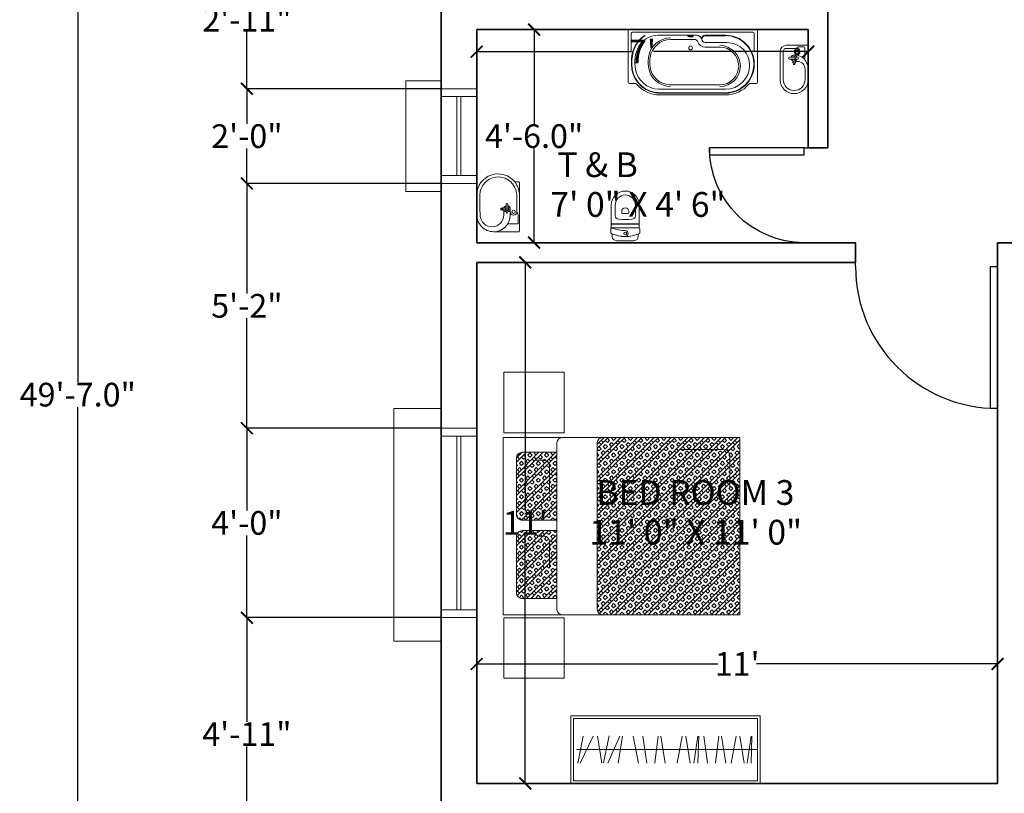
# Model space of a CAD drawing. Units: inches. Extents: x 844 to 2234, y 346 to 1084.
# Tile 48 of 93: x 1590 to 1840, y 632 to 828. Entities that reach past the tile are written whole.
import ezdxf

# ---------------------------------------------------------------- set-up
doc = ezdxf.new("R2010")
doc.units = ezdxf.units.IN
doc.header["$MEASUREMENT"] = 0
for name, color, linetype, lineweight in [('A-ANNO-DIMS', 2, 'Continuous', 18), ('A-AREA-IDEN', 7, 'Continuous', 18), ('A-FLOR-FIXT', 8, 'Continuous', 18), ('A-WALL', 7, 'Continuous', 35), ('beds', 130, 'Continuous', 18), ('doors', 170, 'Continuous', 25), ('furniture', 8, 'Continuous', 18), ('windows', 1, 'Continuous', 18)]:
    doc.layers.add(name, color=color, linetype=linetype, lineweight=lineweight)
doc.styles.get("Standard").update_dxf_attribs({"font": 'arial.ttf'})
doc.dimstyles.get("Standard").update_dxf_attribs({"dimtxt": 6, "dimasz": 3, "dimexe": 0.18, "dimexo": 0.0625, "dimgap": 0.09, "dimtad": 0, "dimtih": 1, "dimtoh": 1, "dimdec": 1, "dimzin": 0, "dimdsep": 46, "dimlunit": 3, "dimtxsty": 'Standard', "dimblk": 'ARCHTICK', "dimcen": 0.09, "dimadec": 0, "dimazin": 0, "dimtfac": 1, "dimtdec": 1, "dimtofl": 0, "dimtmove": 0, "dimatfit": 3, "dimfxl": 1, "dimtolj": 1, "dimtzin": 0, "dimarcsym": 0})
pattern_1 = [(135, (-1377.70473, -125.71507), (-0.070710678, -0.070710678), []), (135, (-1377.68705, -125.69739), (-0.070710678, -0.070710678), []), (45, (-1377.70473, -125.71507), (-0.070710678, 0.070710678), [-0.025, 0.025]), (45, (-1377.72241, -125.69739), (-0.070710678, 0.070710678), [-0.025, 0.025]), (45, (-1377.74009, -125.67972), (-0.070710678, 0.070710678), [0.025, -0.025]), (45, (-1377.75776, -125.66204), (-0.070710678, 0.070710678), [0.025, -0.025]), (135, (-1377.66938, -125.67972), (-0.070710678, -0.070710678), [0.025, -0.025]), (135, (-1377.6517, -125.66204), (-0.070710678, -0.070710678), [0.025, -0.025])]

# ---------------------------------------------------------------- blocks, each defined once
blk = doc.blocks.new('*U2')
for p, q in [((0, 0), (0, -6)), ((36, 0), (36, -6))]:
    blk.add_line(p, q)
blk.add_lwpolyline([(0, 0), (0, 36), (1.75, 36), (1.75, 0)], close=True)
blk.add_arc((0, 0), 36, 0, 90)
blk = doc.blocks.new('*U4')
for p, q in [((0, 0), (0, -6)), ((24, 0), (24, -6))]:
    blk.add_line(p, q)
blk.add_lwpolyline([(0, 0), (0, 24), (1.75, 24), (1.75, 0)], close=True)
blk.add_arc((0, 0), 24, 0, 90)
blk = doc.blocks.new('MAT-P10')
h = blk.add_hatch()
h.set_pattern_fill('BOX', color=256, scale=0.1, angle=45, style=0)
h.set_pattern_definition(pattern_1)
h.paths.add_polyline_path([(-0.1565, 1.4605), (0.417, 1.4605), (0.417, 1.7513, 0.414214), (0.367, 1.8013), (-0.1065, 1.8013, 0.414214), (-0.1565, 1.7513)])
h.paths.add_polyline_path([(0.5052, 1.4604), (1.0792, 1.4604), (1.0792, 1.7513, 0.414214), (1.0292, 1.8013), (0.5552, 1.8013, 0.414214), (0.5052, 1.7513)])
h = blk.add_hatch()
h.set_pattern_fill('BOX', color=256, scale=0.1, angle=45, style=0)
h.set_pattern_definition(pattern_1)
edge = h.paths.add_edge_path()
edge.add_line((1.2049, -0.085), (1.2049, 1.0625))
edge.add_ellipse((1.1608, 1.0627), major_axis=(0, 0.0568), ratio=0.776379, start_angle=270, end_angle=360)
edge.add_line((1.1608, 1.1195), (-0.251, 1.1195))
edge.add_ellipse((-0.251, 1.0627), major_axis=(0, 0.0568), ratio=0.776379, start_angle=0, end_angle=88.13958)
edge.add_line((-0.2951, 1.0641), (-0.2951, -0.085))
edge.add_line((-0.2951, -0.085), (1.2049, -0.085))
for p, q in [((-0.251, 1.4605), (1.1608, 1.4604)), ((-0.251, 1.1195), (1.1608, 1.1195)), ((1.1017, 0.406), (1.1017, 0.0572)), ((1.0576, 0.0004), (0.7754, 0.0004))]:
    blk.add_line(p, q)
for points in [[(1.2049, -0.085), (-0.2951, -0.085), (-0.2951, 1.9151), (1.2049, 1.915)], [(-0.8301, 1.9091), (-0.3191, 1.9091), (-0.3191, 1.3981), (-0.8301, 1.3981)], [(1.2441, 1.9091), (1.755, 1.9091), (1.755, 1.3981), (1.2441, 1.3981)]]:
    blk.add_lwpolyline(points, close=True)
for points in [[(0.417, 1.4604), (0.417, 1.7513, 0.414214), (0.367, 1.8013), (-0.1065, 1.8013, 0.414214), (-0.1565, 1.7513), (-0.1565, 1.4604)], [(1.0792, 1.4603), (1.0792, 1.7513, 0.414214), (1.0292, 1.8013), (0.5552, 1.8013, 0.414214), (0.5052, 1.7513), (0.5052, 1.4604)], [(0.3702, 1.6242), (0.3702, 1.5715, -0.414214), (0.3202, 1.5215), (0.1113, 1.5215)], [(1.0117, 1.6438), (1.0117, 1.5715, -0.414214), (0.9617, 1.5215), (0.7528, 1.5215)]]:
    blk.add_lwpolyline(points, format="xyb")
at = {"extrusion": (0, 0, -1)}
for centre, start_param, end_param in [((-0.251, 1.4036), 4.712389, 6.283185), ((1.1608, 1.4036), 0, 1.570796), ((-0.251, 1.0627), 4.712389, 6.283185), ((1.1608, 1.0627), 0, 1.570796), ((1.0576, 0.0572), 1.570796, 3.141593), ((1.0576, 0.0572), 1.570796, 3.141593)]:
    blk.add_ellipse(centre, major_axis=(0, 0.0568), ratio=0.776379, start_param=start_param, end_param=end_param, dxfattribs=at)
blk = doc.blocks.new('A$C7A17768A')
for p, q in [((-2.8, 0), (0, 0)), ((-2.8, -1), (-2.8, 0)), ((0, -1), (0, 0)), ((-2.76, -0.04), (-0.04, -0.04)), ((-2.76, -0.96), (-2.76, -0.04)), ((-0.04, -0.96), (-0.04, -0.04)), ((-2.617, -0.3), (-2.694, -0.7)), ((-2.66, -0.7), (-2.466, -0.3)), ((-2.403, -0.3), (-2.342, -0.7)), ((-2.229, -0.296), (-2.317, -0.696)), ((-2.074, -0.3), (-2.25, -0.7)), ((-2.096, -0.7), (-2.033, -0.3)), ((-1.875, -0.3), (-1.796, -0.7)), ((-1.732, -0.3), (-1.675, -0.7)), ((-1.555, -0.7), (-1.507, -0.3)), ((-1.467, -0.3), (-1.403, -0.7)), ((-1.227, -0.7), (-1.151, -0.3)), ((-1.098, -0.3), (-1.034, -0.7)), ((-0.98, -0.7), (-0.921, -0.3)), ((-0.908, -0.3), (-0.919, -0.7)), ((-0.834, -0.3), (-0.777, -0.7)), ((-0.657, -0.7), (-0.61, -0.3)), ((-0.57, -0.3), (-0.505, -0.7)), ((-0.429, -0.7), (-0.353, -0.3)), ((-0.301, -0.3), (-0.237, -0.7)), ((-0.192, -0.7), (-0.133, -0.3)), ((-0.12, -0.3), (-0.131, -0.7)), ((-0.04, -0.5), (-2.716, -0.5)), ((-2.8, -1), (0, -1)), ((-2.76, -0.96), (-0.04, -0.96))]:
    blk.add_line(p, q)
blk = doc.blocks.new('2SABICO')
at = {"color": 0, "linetype": 'ByBlock'}
for p, q in [((0.478, 0.195), (0.089, 0.195)), ((0.478, 0.152), (0.089, 0.152)), ((0, 0.106), (0, 0)), ((0, 0), (0, -0.18)), ((0.043, -0.039), (0.043, 0.106)), ((0.135, 0), (0.135, -0.003)), ((0.168, 0.064), (0.168, -0.015)), ((0.192, 0.064), (0.192, -0.015)), ((0.221, 0.012), (0.222, 0.012)), ((0.223, 0.016), (0.223, -0.016)), ((0.224, 0.017), (0.245, 0.017)), ((0.246, 0.016), (0.246, -0.016)), ((0.25, 0.014), (0.246, 0.014)), ((0.26, 0.01), (0.268, 0.01)), ((0.268, -0.01), (0.268, 0.01)), ((0.268, 0.01), (0.269, 0.009)), ((0.269, -0.009), (0.269, 0.009)), ((0.023, -0.057), (0.023, -0.135)), ((0.135, 0), (0.135, -0.039)), ((0.168, -0.015), (0.192, -0.015)), ((0.168, -0.015), (0.168, -0.046)), ((0.192, -0.015), (0.192, -0.046)), ((0.221, -0.012), (0.222, -0.012)), ((0.224, -0.017), (0.245, -0.017)), ((0.225, -0.017), (0.225, -0.047)), ((0.25, -0.014), (0.246, -0.014)), ((0.26, -0.01), (0.268, -0.01)), ((0.268, -0.01), (0.269, -0.009)), ((0.015, -0.195), (0.478, -0.195)), ((0.038, -0.15), (0.179, -0.15)), ((0.33, -0.152), (0.478, -0.152))]:
    blk.add_line(p, q, dxfattribs=at)
for radius in [0.035, 0.023]:
    blk.add_circle((0.089, -0.039), radius, dxfattribs=at)
for centre, radius, start, end in [((0.089, 0.106), 0.089, 90, 180), ((0.089, 0.106), 0.046, 90, 180), ((0.478, 0), 0.195, 270, 90), ((0.478, 0), 0.152, 270, 90), ((0.18, 0), 0.045, 105.6643, 180), ((0.18, 0), 0.042, 106.8152, 252.6853), ((0.18, 0), 0.0235, 121.1327, 237.8651), ((0.18, 0.064), 0.0121, 0, 180), ((0.18, 0), 0.045, 17.0576, 74.3357), ((0.18, 0), 0.042, 287.3147, 73.1848), ((0.18, 0), 0.0235, 302.1349, 58.8673), ((0.221, 0.013), 0.001, 197.9471, 270), ((0.222, 0.013), 0.001, 270, 0), ((0.224, 0.016), 0.001, 90, 180), ((0.245, 0.016), 0.001, 0, 90), ((0.25, 0), 0.0143, 270, 90), ((0.041, -0.057), 0.018, 99.5941, 180), ((0.038, -0.135), 0.015, 180, 270), ((0.037, -0.033), 0.006, 279.5941, 0), ((0.089, -0.039), 0.046, 180, 360), ((0.326, -0.003), 0.191, 180, 270), ((0.18, -0.046), 0.0125, 180, 0), ((0.179, -0.14), 0.01, 270, 42.9682), ((0.221, -0.013), 0.001, 90, 162.0529), ((0.222, -0.013), 0.001, 0, 90), ((0.224, -0.016), 0.001, 180, 270), ((0.33, -0.047), 0.105, 180, 270), ((0.245, -0.016), 0.001, 270, 0), ((0.015, -0.18), 0.015, 180, 270)]:
    blk.add_arc(centre, radius, start, end, dxfattribs=at)
blk = doc.blocks.new('2SAINCO')
at = {"color": 0, "linetype": 'ByBlock'}
for p, q in [((0.06, 0.181), (0.085, 0.181)), ((0.114, 0.203), (0.165, 0.203)), ((0.496, 0.195), (0.178, 0.195)), ((0.18, -0.188), (0.18, 0.188)), ((0.231, 0.185), (0.231, -0.185)), ((0.234, 0.185), (0.234, -0.185)), ((0.496, 0.14), (0.347, 0.14)), ((0, -0.121), (0, 0.121)), ((0.394, 0.05), (0.407, 0.05)), ((0.394, -0.05), (0.407, -0.05)), ((0.06, -0.181), (0.085, -0.181)), ((0.114, -0.201), (0.165, -0.201)), ((0.114, -0.203), (0.165, -0.203)), ((0.496, -0.195), (0.178, -0.195)), ((0.496, -0.14), (0.347, -0.14))]:
    blk.add_line(p, q, dxfattribs=at)
blk.add_circle((0.1, 0), 0.02, dxfattribs=at)
for centre, radius, start, end in [((0.06, 0.121), 0.06, 90, 180), ((0.517, 0), 0.46, 155.909, 204.091), ((0.085, 0.196), 0.015, 270, 344.534), ((0.114, 0.188), 0.015, 90, 164.534), ((0.165, 0.188), 0.015, 0, 90), ((0.221, 0.185), 0.01, 0, 90), ((0.224, 0.185), 0.01, 0, 90), ((0.347, 0.09), 0.05, 90, 177.3546), ((0.496, 0), 0.195, 270, 90), ((0.496, 0), 0.14, 270, 90), ((0.1, 0), 0.0405, 360, 180), ((0.517, 0), 0.458, 180, 204.67), ((0.66, 0.008), 0.52, 180.891, 201.3823), ((2.295, 0), 2, 177.3546, 182.6454), ((0.677, 0), 0.3, 172.9459, 187.0541), ((0.394, 0.035), 0.015, 90, 172.9459), ((0.407, 0), 0.05, 270, 90), ((0.06, -0.121), 0.06, 180, 270), ((0.347, -0.09), 0.05, 182.6454, 270), ((0.394, -0.035), 0.015, 187.0541, 270), ((0.085, -0.196), 0.015, 15.466, 90), ((0.114, -0.188), 0.015, 195.466, 270), ((0.114, -0.188), 0.013, 195.466, 270), ((0.165, -0.188), 0.013, 270, 30), ((0.165, -0.188), 0.015, 270, 0), ((0.221, -0.185), 0.01, 270, 0), ((0.224, -0.185), 0.01, 270, 0)]:
    blk.add_arc(centre, radius, start, end, dxfattribs=at)
blk = doc.blocks.new('2SABACO')
at = {"color": 0}
for p, q in [((1.341, 0.831), (0.407, 0.831)), ((1.341, 0.91), (0.429, 0.91)), ((1.341, 0.885), (0.429, 0.885)), ((1.341, 0.879), (0.429, 0.879)), ((-0.015, 0.735), (-0.015, 0.015)), ((0, 0.75), (0.08, 0.75)), ((1.263, 0.769), (0.562, 0.769)), ((1.77, 0.75), (1.69, 0.75)), ((1.785, 0.015), (1.785, 0.735)), ((0.03, 0.302), (0.03, 0.053)), ((1.74, 0.053), (1.74, 0.286)), ((0.578, 0.139), (0.911, 0.139)), ((1.263, 0.245), (1.06, 0.245)), ((1.363, 0.181), (1.06, 0.181)), ((0, 0), (1.77, 0)), ((0.048, 0.035), (1.722, 0.035)), ((0.401, 0.08), (0.942, 0.08)), ((1.343, 0.086), (1.06, 0.086)), ((1.343, 0.079), (1.06, 0.079))]:
    blk.add_line(p, q, dxfattribs=at)
blk.add_circle((0.855, 0.256), 0.026, dxfattribs=at)
for centre, radius, start, end in [((0.428, 0.49), 0.395, 98.9726, 181.1954), ((0.428, 0.49), 0.389, 98.9726, 181.2301), ((0.425, 0.49), 0.342, 93.1008, 168.0202), ((0.429, 0.48), 0.43, 90, 139.2943), ((0.429, 0.48), 0.405, 90, 98.9726), ((0.429, 0.48), 0.399, 90, 98.9726), ((1.341, 0.48), 0.43, 40.7057, 90), ((1.341, 0.485), 0.401, 359.4627, 90), ((1.341, 0.485), 0.394, 3.5237, 90), ((1.341, 0.495), 0.336, 0, 90), ((0, 0.735), 0.015, 90, 180), ((0.08, 0.78), 0.03, 270, 319.2943), ((0.578, 0.481), 0.311, 90, 172.609), ((0.578, 0.481), 0.288, 93.3767, 172.609), ((1.263, 0.507), 0.285, 270, 90), ((1.263, 0.507), 0.262, 270, 90), ((1.69, 0.78), 0.03, 220.7057, 270), ((1.77, 0.735), 0.015, 0, 90), ((0.559, 0.454), 0.48, 163.1286, 202.3619), ((0.559, 0.454), 0.528, 177.0415, 202.3619), ((0.559, 0.454), 0.521, 177.0156, 202.3619), ((0.79, 0.454), 0.525, 172.609, 180), ((0.79, 0.454), 0.525, 180, 187.391), ((0.79, 0.454), 0.502, 172.609, 180), ((0.79, 0.454), 0.502, 180, 187.391), ((1.343, 0.477), 0.392, 270, 4.5675), ((1.343, 0.477), 0.398, 270, 0.539), ((1.363, 0.495), 0.314, 270, 2.2815), ((0.042, 0.302), 0.0116, 16.3184, 180.0001), ((0.578, 0.427), 0.311, 187.391, 270), ((0.578, 0.427), 0.288, 187.391, 270), ((1.718, 0.286), 0.0222, 0, 152.9966), ((0.401, 0.389), 0.357, 202.3619, 239.8287), ((0.401, 0.389), 0.351, 202.3619, 239.2093), ((0.401, 0.389), 0.309, 202.3619, 270), ((0.911, 0.183), 0.045, 270, 341.2369), ((1.06, 0.133), 0.112, 90, 161.2369), ((1.06, 0.133), 0.0475, 90, 270), ((0, 0.015), 0.015, 180, 270), ((0.048, 0.053), 0.018, 180, 270), ((0.559, 0.454), 0.48, 250.7818, 251.0555), ((0.821, 0.092), 0.00282, 119.7759, 180), ((0.821, 0.092), 0.00282, 180, 240.2241), ((0.837, 0.064), 0.0347, 103.3326, 119.7759), ((0.835, 0.025), 0.071, 96.5949, 102.1924), ((0.837, 0.12), 0.0347, 240.2241, 256.6674), ((0.847, -0.08), 0.177, 92.7417, 96.5949), ((0.848, 0.02), 0.0808, 95.6065, 103.3326), ((0.848, 0.164), 0.0808, 256.6674, 264.3935), ((0.855, -0.252), 0.349, 90, 92.7417), ((0.855, -0.053), 0.153, 90, 95.6065), ((0.855, 0.237), 0.153, 264.3935, 270), ((0.855, -0.053), 0.153, 84.3935, 90), ((0.855, -0.252), 0.349, 87.2583, 90), ((0.855, 0.237), 0.153, 270, 275.6065), ((0.862, 0.02), 0.0808, 76.6674, 84.3935), ((0.862, 0.164), 0.0808, 275.6065, 283.3326), ((0.863, -0.08), 0.177, 83.4051, 87.2583), ((0.873, 0.064), 0.0347, 60.2241, 76.6674), ((0.873, 0.12), 0.0347, 283.3326, 299.7759), ((0.875, 0.025), 0.071, 77.8076, 83.4051), ((0.889, 0.092), 0.00282, 360, 60.2241), ((0.889, 0.092), 0.00282, 299.7759, 360), ((0.942, 0.145), 0.065, 270, 349.4977), ((1.06, 0.133), 0.054, 180, 270), ((1.722, 0.053), 0.018, 270, 0), ((1.77, 0.015), 0.015, 270, 0)]:
    blk.add_arc(centre, radius, start, end, dxfattribs=at)
blk = doc.blocks.new('2SALACO2')
at = {"color": 0}
for p, q in [((0, 0), (-0.392, 0)), ((0.28, 0), (0, 0)), ((-0.402, -0.01), (-0.402, -0.36)), ((-0.293, -0.026), (-0.293, -0.15)), ((-0.283, -0.016), (-0.166, -0.016)), ((-0.169, -0.128), (-0.085, -0.128)), ((-0.112, -0.035), (-0.133, -0.035)), ((-0.124, -0.035), (0.09, -0.035)), ((0.29, -0.01), (0.29, -0.064)), ((-0.102, -0.219), (-0.169, -0.219)), ((-0.1, -0.161), (-0.131, -0.161)), ((-0.1, -0.186), (-0.131, -0.186)), ((-0.102, -0.217), (-0.102, -0.234)), ((-0.07, -0.216), (-0.101, -0.216)), ((-0.07, -0.235), (-0.101, -0.235)), ((-0.1, -0.161), (-0.1, -0.186)), ((-0.021, -0.161), (-0.1, -0.161)), ((-0.021, -0.186), (-0.1, -0.186)), ((-0.098, -0.214), (-0.098, -0.216)), ((-0.097, -0.239), (-0.098, -0.241)), ((-0.098, -0.241), (-0.098, -0.248)), ((-0.098, -0.241), (-0.073, -0.241)), ((-0.073, -0.248), (-0.098, -0.248)), ((-0.097, -0.235), (-0.097, -0.239)), ((-0.074, -0.239), (-0.097, -0.239)), ((-0.097, -0.248), (-0.097, -0.256)), ((-0.073, -0.256), (-0.097, -0.256)), ((-0.097, -0.256), (-0.094, -0.257)), ((-0.077, -0.257), (-0.094, -0.257)), ((-0.073, -0.256), (-0.077, -0.257)), ((-0.074, -0.235), (-0.074, -0.239)), ((-0.074, -0.239), (-0.073, -0.241)), ((-0.073, -0.214), (-0.073, -0.216)), ((-0.073, -0.241), (-0.073, -0.248)), ((-0.073, -0.248), (-0.073, -0.256)), ((-0.069, -0.217), (-0.069, -0.234))]:
    blk.add_line(p, q, dxfattribs=at)
blk.add_lwpolyline([(-0.402, -0.36, 0.423787), (-0.161, -0.593, 0.423787)], format="xyb", dxfattribs=at)
blk.add_circle((-0.124, -0.081), 0.023, dxfattribs=at)
for centre, radius, start, end in [((-0.392, -0.01), 0.01, 90, 180), ((0.28, -0.01), 0.01, 0, 90), ((-0.169, -0.36), 0.233, 90, 180), ((-0.283, -0.026), 0.01, 90, 180), ((-0.124, -0.081), 0.0462, 90, 270), ((-0.166, -0.046), 0.03, 31.2573, 90), ((-0.133, -0.026), 0.009, 211.2573, 270), ((-0.085, -0.173), 0.042, 16.8152, 162.6853), ((-0.085, -0.173), 0.0458, 15.3964, 90), ((0.09, -0.29), 0.255, 68.9449, 90), ((0.105, -0.295), 0.255, 271.0077, 72.4499), ((0.105, -0.297), 0.297, 271.4871, 51.4524), ((0.105, -0.297), 0.297, 51.4524, 87.1707), ((-0.169, -0.383), 0.164, 90, 265.4963), ((-0.285, -0.15), 0.008, 180, 299.1062), ((-0.131, -0.173), 0.0125, 90, 270), ((-0.085, -0.173), 0.042, 197.3147, 343.1848), ((-0.085, -0.173), 0.0235, 31.1327, 147.8651), ((-0.085, -0.173), 0.0235, 212.1349, 328.8673), ((-0.101, -0.217), 0.001, 90, 180), ((-0.101, -0.234), 0.001, 180, 270), ((-0.085, -0.173), 0.0458, 289.9182, 344.6036), ((-0.07, -0.217), 0.001, 0, 90), ((-0.07, -0.234), 0.001, 270, 0), ((-0.021, -0.173), 0.0121, 270, 90), ((0.021, 4.449), 5, 267.6742, 271.0081), ((-0.017, 4.405), 5, 268.3511, 271.4874)]:
    blk.add_arc(centre, radius, start, end, dxfattribs=at)
blk = doc.blocks.new('_ArchTick')
at = {"color": 0, "linetype": 'ByBlock', "const_width": 0.15}
blk.add_lwpolyline([(-0.5, -0.5), (0.5, 0.5)], dxfattribs=at)
blk = doc.blocks.new('*D67')
at = {"layer": 'A-ANNO-DIMS', "color": 0, "lineweight": -2, "transparency": 16777216}
for p, q in [((1714.3, 766.46), (1718.59, 766.46)), ((1718.41, 766.46), (1718.41, 703.56)), ((1718.41, 634.46), (1718.41, 697.35)), ((1714.3, 634.46), (1718.59, 634.46))]:
    blk.add_line(p, q, dxfattribs=at)
at = {"layer": 'Defpoints', "color": 0, "transparency": 16777216}
for p in [(1714.24, 766.46), (1714.24, 634.46), (1718.41, 634.46)]:
    blk.add_point(p, dxfattribs=at)
at = {"layer": 'A-ANNO-DIMS', "color": 0, "lineweight": -2, "transparency": 16777216, "xscale": 3, "yscale": 3, "zscale": 3}
for p, rotation in [((1718.41, 766.46), 90), ((1718.41, 634.46), 270)]:
    blk.add_blockref('_ArchTick', p, dxfattribs=dict(at, rotation=rotation))
at = {"layer": 'A-ANNO-DIMS', "color": 0, "transparency": 16777216, "insert": (1718.41, 700.46), "char_height": 6, "attachment_point": 5}
blk.add_mtext("\\A1;11'", dxfattribs=at)
blk = doc.blocks.new('*D68')
at = {"layer": 'A-ANNO-DIMS', "color": 0, "lineweight": -2, "transparency": 16777216}
for p, q in [((1706.1, 664.78), (1706.1, 664.9)), ((1706.1, 664.72), (1767.2, 664.72)), ((1838.1, 664.72), (1777, 664.72)), ((1838.1, 664.78), (1838.1, 664.9))]:
    blk.add_line(p, q, dxfattribs=at)
at = {"layer": 'Defpoints', "color": 0, "transparency": 16777216}
for p in [(1706.1, 664.72), (1838.1, 664.72), (1838.1, 664.72)]:
    blk.add_point(p, dxfattribs=at)
at = {"layer": 'A-ANNO-DIMS', "color": 0, "lineweight": -2, "transparency": 16777216, "xscale": 3, "yscale": 3, "zscale": 3, "rotation": 180}
blk.add_blockref('_ArchTick', (1706.1, 664.72), dxfattribs=at)
at = {"layer": 'A-ANNO-DIMS', "color": 0, "lineweight": -2, "transparency": 16777216, "xscale": 3, "yscale": 3, "zscale": 3}
blk.add_blockref('_ArchTick', (1838.1, 664.72), dxfattribs=at)
at = {"layer": 'A-ANNO-DIMS', "color": 0, "transparency": 16777216, "insert": (1772.1, 664.72), "char_height": 6, "attachment_point": 5}
blk.add_mtext("\\A1;11'", dxfattribs=at)
blk = doc.blocks.new('*D63')
at = {"layer": 'A-ANNO-DIMS', "color": 0, "lineweight": -2, "transparency": 16777216}
for p, q in [((1733.04, 825.46), (1720.47, 825.46)), ((1720.65, 825.46), (1720.65, 801.61)), ((1720.65, 771.46), (1720.65, 795.3)), ((1733.04, 771.46), (1720.47, 771.46))]:
    blk.add_line(p, q, dxfattribs=at)
at = {"layer": 'Defpoints', "color": 0, "transparency": 16777216}
for p in [(1733.1, 825.46), (1720.65, 771.46), (1733.1, 771.46)]:
    blk.add_point(p, dxfattribs=at)
at = {"layer": 'A-ANNO-DIMS', "color": 0, "lineweight": -2, "transparency": 16777216, "xscale": 3, "yscale": 3, "zscale": 3}
for p, rotation in [((1720.65, 825.46), 90), ((1720.65, 771.46), 270)]:
    blk.add_blockref('_ArchTick', p, dxfattribs=dict(at, rotation=rotation))
at = {"layer": 'A-ANNO-DIMS', "color": 0, "transparency": 16777216, "insert": (1720.65, 798.46), "char_height": 6, "attachment_point": 5}
blk.add_mtext('\\A1;4\'-6.0"', dxfattribs=at)
blk = doc.blocks.new('*D64')
at = {"layer": 'A-ANNO-DIMS', "color": 0, "lineweight": -2, "transparency": 16777216}
for p, q in [((1706.1, 823.41), (1706.1, 819.69)), ((1790.1, 823.41), (1790.1, 819.69)), ((1706.1, 819.87), (1745.27, 819.87)), ((1790.1, 819.87), (1750.93, 819.87))]:
    blk.add_line(p, q, dxfattribs=at)
at = {"layer": 'Defpoints', "color": 0, "transparency": 16777216}
for p in [(1706.1, 823.47), (1790.1, 823.47), (1706.1, 819.87)]:
    blk.add_point(p, dxfattribs=at)
at = {"layer": 'A-ANNO-DIMS', "color": 0, "lineweight": -2, "transparency": 16777216, "xscale": 3, "yscale": 3, "zscale": 3, "rotation": 180}
blk.add_blockref('_ArchTick', (1706.1, 819.87), dxfattribs=at)
at = {"layer": 'A-ANNO-DIMS', "color": 0, "lineweight": -2, "transparency": 16777216, "xscale": 3, "yscale": 3, "zscale": 3}
blk.add_blockref('_ArchTick', (1790.1, 819.87), dxfattribs=at)
at = {"layer": 'A-ANNO-DIMS', "color": 0, "transparency": 16777216, "insert": (1748.1, 819.87), "char_height": 6, "attachment_point": 5}
blk.add_mtext("\\A1;7'", dxfattribs=at)
blk = doc.blocks.new('*D87')
at = {"layer": 'A-ANNO-DIMS', "color": 0, "lineweight": -2, "transparency": 16777216}
for p, q in [((1697.04, 1030.46), (1604.81, 1030.46)), ((1604.99, 1030.46), (1604.99, 736.11)), ((1604.99, 435.46), (1604.99, 729.8)), ((1697.04, 435.46), (1604.81, 435.46))]:
    blk.add_line(p, q, dxfattribs=at)
at = {"layer": 'Defpoints', "color": 0, "transparency": 16777216}
for p in [(1697.1, 1030.46), (1604.99, 435.46), (1697.1, 435.46)]:
    blk.add_point(p, dxfattribs=at)
at = {"layer": 'A-ANNO-DIMS', "color": 0, "lineweight": -2, "transparency": 16777216, "xscale": 3, "yscale": 3, "zscale": 3}
for p, rotation in [((1604.99, 1030.46), 90), ((1604.99, 435.46), 270)]:
    blk.add_blockref('_ArchTick', p, dxfattribs=dict(at, rotation=rotation))
at = {"layer": 'A-ANNO-DIMS', "color": 0, "transparency": 16777216, "insert": (1604.99, 732.96), "char_height": 6, "attachment_point": 5}
blk.add_mtext('\\A1;49\'-7.0"', dxfattribs=at)
blk = doc.blocks.new('WIN-48IN')
for p, q in [((0, 9), (0, 21)), ((0, 21), (59, 21)), ((59, 9), (59, 21)), ((6, 9), (0, 9)), ((54, 9), (6, 9)), ((6, 9), (6, 0)), ((8, 9), (8, 0)), ((52, 0), (52, 9)), ((54, 0), (54, 9)), ((54, 9), (59, 9)), ((8, 5), (52, 5)), ((8, 4), (52, 4)), ((6, 0), (54, 0))]:
    blk.add_line(p, q)
blk = doc.blocks.new('WIN-24IN')
for p, q in [((9, 28), (0, 28)), ((0, 0), (0, 28)), ((9, 26), (9, 28)), ((18, 26), (9, 26)), ((9, 26), (9, 2)), ((18, 2), (18, 26)), ((18, 24), (9, 24)), ((13, 4), (13, 24)), ((14, 4), (14, 24)), ((9, 4), (18, 4)), ((9, 2), (18, 2)), ((9, 2), (9, 0)), ((9, 0), (0, 0))]:
    blk.add_line(p, q)
blk = doc.blocks.new('*D163')
at = {"layer": 'A-ANNO-DIMS', "color": 0, "lineweight": -2, "transparency": 16777216}
for p, q in [((1697.04, 676.46), (1647.67, 676.46)), ((1647.85, 676.46), (1647.85, 650.06)), ((1647.85, 617.46), (1647.85, 643.85)), ((1697.04, 617.46), (1647.67, 617.46))]:
    blk.add_line(p, q, dxfattribs=at)
at = {"layer": 'Defpoints', "color": 0, "transparency": 16777216}
for p in [(1647.85, 676.46), (1697.1, 676.46), (1697.1, 617.46)]:
    blk.add_point(p, dxfattribs=at)
at = {"layer": 'A-ANNO-DIMS', "color": 0, "lineweight": -2, "transparency": 16777216, "xscale": 3, "yscale": 3, "zscale": 3}
for p, rotation in [((1647.85, 676.46), 90), ((1647.85, 617.46), 270)]:
    blk.add_blockref('_ArchTick', p, dxfattribs=dict(at, rotation=rotation))
at = {"layer": 'A-ANNO-DIMS', "color": 0, "transparency": 16777216, "insert": (1647.85, 646.96), "char_height": 6, "attachment_point": 5}
blk.add_mtext('\\A1;4\'-11"', dxfattribs=at)
blk = doc.blocks.new('*D164')
at = {"layer": 'A-ANNO-DIMS', "color": 0, "lineweight": -2, "transparency": 16777216}
for p, q in [((1697.04, 724.46), (1647.67, 724.46)), ((1647.85, 724.46), (1647.85, 703.61)), ((1647.85, 676.46), (1647.85, 697.3)), ((1697.04, 676.46), (1647.67, 676.46))]:
    blk.add_line(p, q, dxfattribs=at)
at = {"layer": 'Defpoints', "color": 0, "transparency": 16777216}
for p in [(1647.85, 724.46), (1697.1, 724.46), (1697.1, 676.46)]:
    blk.add_point(p, dxfattribs=at)
at = {"layer": 'A-ANNO-DIMS', "color": 0, "lineweight": -2, "transparency": 16777216, "xscale": 3, "yscale": 3, "zscale": 3}
for p, rotation in [((1647.85, 724.46), 90), ((1647.85, 676.46), 270)]:
    blk.add_blockref('_ArchTick', p, dxfattribs=dict(at, rotation=rotation))
at = {"layer": 'A-ANNO-DIMS', "color": 0, "transparency": 16777216, "insert": (1647.85, 700.46), "char_height": 6, "attachment_point": 5}
blk.add_mtext('\\A1;4\'-0"', dxfattribs=at)
blk = doc.blocks.new('*D165')
at = {"layer": 'A-ANNO-DIMS', "color": 0, "lineweight": -2, "transparency": 16777216}
for p, q in [((1697.04, 786.46), (1647.67, 786.46)), ((1647.85, 786.46), (1647.85, 758.61)), ((1647.85, 724.46), (1647.85, 752.3)), ((1697.04, 724.46), (1647.67, 724.46))]:
    blk.add_line(p, q, dxfattribs=at)
at = {"layer": 'Defpoints', "color": 0, "transparency": 16777216}
for p in [(1647.85, 786.46), (1697.1, 786.46), (1697.1, 724.46)]:
    blk.add_point(p, dxfattribs=at)
at = {"layer": 'A-ANNO-DIMS', "color": 0, "lineweight": -2, "transparency": 16777216, "xscale": 3, "yscale": 3, "zscale": 3}
for p, rotation in [((1647.85, 786.46), 90), ((1647.85, 724.46), 270)]:
    blk.add_blockref('_ArchTick', p, dxfattribs=dict(at, rotation=rotation))
at = {"layer": 'A-ANNO-DIMS', "color": 0, "transparency": 16777216, "insert": (1647.85, 755.46), "char_height": 6, "attachment_point": 5}
blk.add_mtext('\\A1;5\'-2"', dxfattribs=at)
blk = doc.blocks.new('*D166')
at = {"layer": 'A-ANNO-DIMS', "color": 0, "lineweight": -2, "transparency": 16777216}
for p, q in [((1697.04, 810.46), (1647.67, 810.46)), ((1647.85, 810.46), (1647.85, 801.61)), ((1647.85, 786.46), (1647.85, 795.3)), ((1697.04, 786.46), (1647.67, 786.46))]:
    blk.add_line(p, q, dxfattribs=at)
at = {"layer": 'Defpoints', "color": 0, "transparency": 16777216}
for p in [(1647.85, 810.46), (1697.1, 810.46), (1697.1, 786.46)]:
    blk.add_point(p, dxfattribs=at)
at = {"layer": 'A-ANNO-DIMS', "color": 0, "lineweight": -2, "transparency": 16777216, "xscale": 3, "yscale": 3, "zscale": 3}
for p, rotation in [((1647.85, 810.46), 90), ((1647.85, 786.46), 270)]:
    blk.add_blockref('_ArchTick', p, dxfattribs=dict(at, rotation=rotation))
at = {"layer": 'A-ANNO-DIMS', "color": 0, "transparency": 16777216, "insert": (1647.85, 798.46), "char_height": 6, "attachment_point": 5}
blk.add_mtext('\\A1;2\'-0"', dxfattribs=at)
blk = doc.blocks.new('*D167')
at = {"layer": 'A-ANNO-DIMS', "color": 0, "lineweight": -2, "transparency": 16777216}
for p, q in [((1697.04, 845.46), (1647.67, 845.46)), ((1647.85, 845.46), (1647.85, 831.06)), ((1647.85, 810.46), (1647.85, 824.85)), ((1697.04, 810.46), (1647.67, 810.46))]:
    blk.add_line(p, q, dxfattribs=at)
at = {"layer": 'Defpoints', "color": 0, "transparency": 16777216}
for p in [(1647.85, 845.46), (1697.1, 845.46), (1697.1, 810.46)]:
    blk.add_point(p, dxfattribs=at)
at = {"layer": 'A-ANNO-DIMS', "color": 0, "lineweight": -2, "transparency": 16777216, "xscale": 3, "yscale": 3, "zscale": 3}
for p, rotation in [((1647.85, 845.46), 90), ((1647.85, 810.46), 270)]:
    blk.add_blockref('_ArchTick', p, dxfattribs=dict(at, rotation=rotation))
at = {"layer": 'A-ANNO-DIMS', "color": 0, "transparency": 16777216, "insert": (1647.85, 827.96), "char_height": 6, "attachment_point": 5}
blk.add_mtext('\\A1;2\'-11"', dxfattribs=at)

msp = doc.modelspace()

# ---------------------------------------------------------------- linework, layer by layer
at = {"layer": 'A-WALL'}
for p, q in [((1697.1, 1030.46), (1697.1, 435.46)), ((1795.1, 884.46), (1795.1, 795.46)), ((1706.1, 825.46), (1706.1, 771.46)), ((1706.1, 825.46), (1790.1, 825.46)), ((1790.1, 825.46), (1790.1, 795.46)), ((1795.1, 795.46), (1790.1, 795.46)), ((1706.1, 771.46), (1790.1, 771.46)), ((1795.1, 771.46), (1790.1, 771.46)), ((1795.1, 771.46), (1802.1, 771.46)), ((1802.1, 766.46), (1802.1, 771.46)), ((1838.1, 771.46), (1843.1, 771.46)), ((1838.1, 766.46), (1838.1, 771.46)), ((1706.1, 766.46), (1706.1, 634.46)), ((1706.1, 766.46), (1802.1, 766.46)), ((1838.1, 766.46), (1838.1, 634.46)), ((1706.1, 634.46), (1838.1, 634.46))]:
    msp.add_line(p, q, dxfattribs=at)

# ---------------------------------------------------------------- block references
at = {"layer": 'A-FLOR-FIXT', "xscale": -18.21101258924898, "yscale": 18.21101258924898, "zscale": 18.21101258924898}
for name, p, rotation in [('2SABACO', (1744.73, 825.46), 180), ('2SABICO', (1786.55, 821.48), 90), ('2SALACO2', (1716.92, 781.56), 270), ('2SAINCO', (1743.76, 771.97), 270)]:
    msp.add_blockref(name, p, dxfattribs=dict(at, rotation=rotation))
at = {"layer": 'beds', "xscale": 29.99962925113936, "yscale": 29.99962925113936, "zscale": 29.99962925113936, "rotation": 90}
msp.add_blockref('MAT-P10', (1770.23, 685.99), dxfattribs=at)
at = {"layer": 'doors', "xscale": -1, "rotation": 90}
msp.add_blockref('*U4', (1789.1, 795.46), dxfattribs=at)
at = {"layer": 'doors', "rotation": 180}
msp.add_blockref('*U2', (1838.1, 765.46), dxfattribs=at)
at = {"layer": 'furniture', "xscale": 17.14285714285603, "yscale": 17.14285714285603, "zscale": 17.14285714285603}
msp.add_blockref('A$C7A17768A', (1777.92, 651.6), dxfattribs=at)
at = {"layer": 'windows'}
msp.add_blockref('WIN-24IN', (1688.1, 784.46), dxfattribs=at)
at = {"layer": 'windows', "rotation": 90.00000000000163}
msp.add_blockref('WIN-48IN', (1706.1, 670.46), dxfattribs=at)

# ---------------------------------------------------------------- texts
at = {"layer": 'A-AREA-IDEN'}
for s, height, p in [('T & B', 6.269, (1726.54, 788.08)), (' 7\' 0" X 4\' 6"', 6.2688, (1722.84, 778.01)), ('BED ROOM 3', 6.269, (1736.43, 705.04)), (' 11\' 0" X 11\' 0"', 6.2688, (1732.74, 694.97))]:
    msp.add_text(s, height=height, dxfattribs=at).set_placement(p)

# ---------------------------------------------------------------- dimensions: what is measured, and where the dimension line sits
at = {"layer": 'A-ANNO-DIMS'}
for base, p1, p2, override, picture, middle in [((1604.99, 435.46), (1697.1, 1030.46), (1697.1, 435.46), {"dimclrd": 0, "dimclre": 0, "dimclrt": 0}, '*D87', (1604.99, 732.96)), ((1647.85, 845.46), (1697.1, 810.46), (1697.1, 845.46), {"dimdec": 1, "dimlfac": 1, "dimrnd": 0, "dimzin": 1, "dimdsep": 46, "dimlunit": 4, "dimfrac": 2}, '*D167', (1647.85, 827.96)), ((1720.65, 771.46), (1733.1, 825.46), (1733.1, 771.46), {"dimclrd": 0, "dimclre": 0, "dimclrt": 0}, '*D63', (1720.65, 798.46)), ((1647.85, 810.46), (1697.1, 786.46), (1697.1, 810.46), {"dimdec": 1, "dimlfac": 1, "dimrnd": 0, "dimzin": 1, "dimdsep": 46, "dimlunit": 4, "dimfrac": 2}, '*D166', (1647.85, 798.46)), ((1647.85, 786.46), (1697.1, 724.46), (1697.1, 786.46), {"dimdec": 1, "dimlfac": 1, "dimrnd": 0, "dimzin": 1, "dimdsep": 46, "dimlunit": 4, "dimfrac": 2}, '*D165', (1647.85, 755.46)), ((1718.41, 634.46), (1714.24, 766.46), (1714.24, 634.46), {"dimclrd": 0, "dimclre": 0, "dimclrt": 0}, '*D67', (1718.41, 700.46)), ((1647.85, 724.46), (1697.1, 676.46), (1697.1, 724.46), {"dimdec": 1, "dimlfac": 1, "dimrnd": 0, "dimzin": 1, "dimdsep": 46, "dimlunit": 4, "dimfrac": 2}, '*D164', (1647.85, 700.46)), ((1647.85, 676.46), (1697.1, 617.46), (1697.1, 676.46), {"dimdec": 1, "dimlfac": 1, "dimrnd": 0, "dimzin": 1, "dimdsep": 46, "dimlunit": 4, "dimfrac": 2}, '*D163', (1647.85, 646.96))]:
    dim = msp.add_linear_dim(base=base, p1=p1, p2=p2, angle=90, dimstyle='Standard', override=override, dxfattribs=at)
    dim.commit()
    dim.dimension.update_dxf_attribs({"geometry": picture, "text_midpoint": middle})
for base, p1, p2, picture, middle in [((1706.1, 819.87), (1790.1, 823.47), (1706.1, 823.47), '*D64', (1748.1, 819.87)), ((1838.1, 664.72), (1706.1, 664.72), (1838.1, 664.72), '*D68', (1772.1, 664.72))]:
    dim = msp.add_linear_dim(base=base, p1=p1, p2=p2, dimstyle='Standard', override={"dimclrd": 0, "dimclre": 0, "dimclrt": 0}, dxfattribs=at)
    dim.commit()
    dim.dimension.update_dxf_attribs({"geometry": picture, "text_midpoint": middle})

doc.saveas('drawing.dxf')
